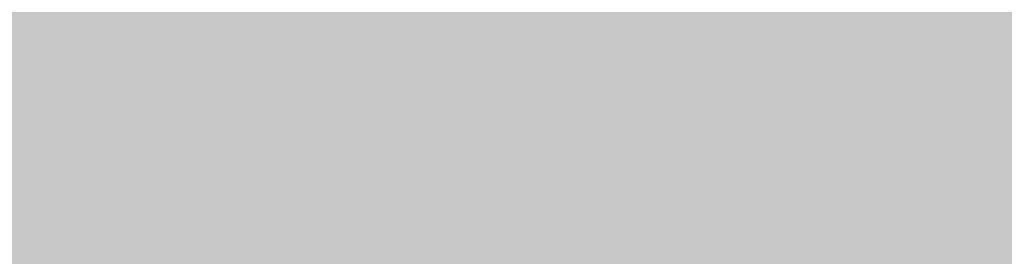
# Model space of a CAD drawing. Units: inches. Extents: x 2083 to 3317, y 1141 to 2115.
# Tile 130 of 256: x 3119.674 to 3123.979, y 1264.131 to 1265.165. Entities that reach past the tile are written whole.
import ezdxf

# ---------------------------------------------------------------- set-up
doc = ezdxf.new("R2010")
doc.units = ezdxf.units.IN
doc.layers.add('A-ANNO-DIMS', color=2, linetype='Continuous', lineweight=18)
doc.layers.add('A-WALL-PATT', color=251, linetype='Continuous', lineweight=13, true_color=0x636466)
doc.styles.get("Standard").update_dxf_attribs({"font": 'arial.ttf'})
doc.dimstyles.new('ISO-25', dxfattribs={"dimtxt": 12, "dimasz": 12, "dimexe": 1.25, "dimexo": 0.625, "dimtad": 1, "dimlunit": 3, "dimtxsty": 'Standard', "dimcen": 2.5, "dimadec": 0, "dimazin": 0, "dimtfac": 1, "dimtmove": 0, "dimatfit": 3, "dimfxl": 1, "dimarcsym": 0})

# ---------------------------------------------------------------- blocks, each defined once
blk = doc.blocks.new('*D26')
at = {"layer": 'A-ANNO-DIMS', "color": 0, "lineweight": -2, "transparency": 16777216}
for p, q in [((3088.9858, 1274.9151), (3088.9858, 1270.952)), ((3111.24, 1274.9151), (3111.24, 1270.952)), ((3076.9858, 1272.202), (2840.2624, 1272.202)), ((3111.24, 1272.202), (3088.9858, 1272.202)), ((3123.24, 1272.202), (3135.24, 1272.202))]:
    blk.add_line(p, q, dxfattribs=at)
at = {"layer": 'A-ANNO-DIMS', "color": 0, "transparency": 16777216}
for points in [[(3076.9858, 1274.202), (3076.9858, 1270.202), (3088.9858, 1272.202)], [(3123.24, 1274.202), (3123.24, 1270.202), (3111.24, 1272.202)]]:
    blk.add_solid(points, dxfattribs=at)
at = {"layer": 'Defpoints', "color": 0, "transparency": 16777216}
for p in [(3088.9858, 1275.5401), (3111.24, 1275.5401), (3088.9858, 1272.202)]:
    blk.add_point(p, dxfattribs=at)
at = {"layer": 'A-ANNO-DIMS', "color": 0, "transparency": 16777216, "insert": (2952.6241, 1279.0316), "char_height": 12, "attachment_point": 5}
blk.add_mtext('NIGHTSTAND 1\'-10 1/2" TYP.', dxfattribs=at)
blk = doc.blocks.new('*D27')
at = {"layer": 'A-ANNO-DIMS', "color": 0, "lineweight": -2, "transparency": 16777216}
for p, q in [((3114.5782, 1309.7943), (3114.5782, 1321.7943)), ((3111.865, 1297.7943), (3115.8282, 1297.7943)), ((3114.5782, 1297.7943), (3114.5782, 1275.5401)), ((3111.865, 1275.5401), (3115.8282, 1275.5401)), ((3114.5782, 1263.5401), (3114.5782, 1140.9886))]:
    blk.add_line(p, q, dxfattribs=at)
at = {"layer": 'A-ANNO-DIMS', "color": 0, "transparency": 16777216}
for points in [[(3112.5782, 1309.7943), (3116.5782, 1309.7943), (3114.5782, 1297.7943)], [(3112.5782, 1263.5401), (3116.5782, 1263.5401), (3114.5782, 1275.5401)]]:
    blk.add_solid(points, dxfattribs=at)
at = {"layer": 'Defpoints', "color": 0, "transparency": 16777216}
for p in [(3111.24, 1297.7943), (3111.24, 1275.5401), (3114.5782, 1275.5401)]:
    blk.add_point(p, dxfattribs=at)
at = {"layer": 'A-ANNO-DIMS', "color": 0, "transparency": 16777216, "insert": (3107.7485, 1196.2643), "char_height": 12, "attachment_point": 5, "rotation": 90}
blk.add_mtext('1\'-10 1/2" TYP.', dxfattribs=at)

msp = doc.modelspace()

# ---------------------------------------------------------------- hatches: boundary and pattern name
at = {"layer": 'A-WALL-PATT'}
h = msp.add_hatch(color=256, dxfattribs=at)
h.dxf.hatch_style = 1
h.paths.add_polyline_path([(3126.9598, 2020.7614), (2748.9598, 2020.7614), (2604.9598, 2020.7614), (2226.9598, 2020.7614), (2226.9598, 1702.7614), (2466.9598, 1702.7614), (2466.9598, 1582.7614), (2418.9598, 1582.7614), (2418.9598, 1477.7614), (2226.9598, 1477.7614), (2226.9598, 1263.2614), (2544.9598, 1263.2614), (2544.9598, 1411.7614), (2604.9598, 1411.7614), (2685.9598, 1411.7614), (2685.9598, 1420.7614), (2604.9598, 1420.7614), (2604.9598, 1573.7614), (2604.9598, 1702.7614), (2604.9598, 2011.7614), (2748.9598, 2011.7614), (2748.9598, 1702.7614), (2862.9598, 1702.7614), (2862.9598, 1621.7614), (2871.9598, 1621.7614), (2871.9598, 1702.7614), (2883.9598, 1702.7614), (2883.9598, 1706.9395, -0.026459), (2883.9598, 1711.7614), (2757.9598, 1711.7614), (2757.9598, 1807.7614), (2787.9598, 1807.7614), (2787.9598, 1812.2614), (2757.9598, 1812.2614), (2757.9598, 2011.7614), (2877.9598, 2011.7614), (2877.9598, 1812.2614), (2847.9598, 1812.2614), (2847.9598, 1807.7614), (2889.8357, 1807.7614), (2889.8357, 1812.2614), (2882.4598, 1812.2614), (2882.4598, 2011.7614), (3117.9598, 2011.7614), (3117.9598, 1812.2614), (2937.8357, 1812.2614), (2937.8357, 1807.7614), (2995.7098, 1807.7614), (2995.7098, 1796.1177), (3000.2098, 1796.1177), (3000.2098, 1807.7614), (3117.9598, 1807.7614), (3117.9598, 1711.7614), (3000.2098, 1711.7614), (3000.2098, 1760.1177), (2998.5727, 1760.1177, -0.020711), (2995.7098, 1760.1177), (2995.7098, 1711.7614), (2931.9598, 1711.7614), (2931.9598, 1702.7614), (3126.9598, 1702.7614)])
h.paths.add_polyline_path([(2471.4598, 2011.7614), (2471.4598, 1810.0114), (2462.7169, 1810.0114), (2462.7169, 1805.5114), (2505.9598, 1805.5114), (2505.9598, 1810.0114), (2475.9598, 1810.0114), (2475.9598, 2011.7614), (2595.9598, 2011.7614), (2595.9598, 1810.0114), (2565.9598, 1810.0114), (2565.9598, 1805.5114), (2595.9598, 1805.5114), (2595.9598, 1711.7614), (2235.9598, 1711.7614), (2235.9598, 1805.5114), (2353.7098, 1805.5114), (2353.7098, 1796.0542), (2358.2098, 1796.0542), (2358.2098, 1805.5114), (2414.7169, 1805.5114), (2414.7169, 1810.0114), (2235.9598, 1810.0114), (2235.9598, 2011.7614)], flags=16)
h.paths.add_polyline_path([(2270.2047, 1994.61), (2270.2047, 1970.61), (2246.2047, 1970.61), (2246.2047, 1994.61)], flags=0)
edge = h.paths.add_edge_path(flags=0)
edge.add_ellipse((2332.0274, 1899.7982), major_axis=(-3.043, 3.043), ratio=0.168252, start_angle=-161.3322, end_angle=-156.3071, ccw=False)
edge.add_ellipse((2333.082, 1898.7435), major_axis=(-1.0546, 1.0546), ratio=0.453532, start_angle=-123.371, end_angle=-94.1591)
edge = h.paths.add_edge_path(flags=0)
edge.add_ellipse((2332.0274, 1968.8763), major_axis=(3.043, 3.043), ratio=0.168252, start_angle=18.6678, end_angle=23.6929)
edge.add_spline(control_points=[(2332.9256, 1970.6911), (2332.2268, 1970.3361), (2330.8937, 1969.6589), (2328.4131, 1970.9321), (2327.2039, 1967.7487), (2324.7096, 1969.9556), (2322.5328, 1967.0124), (2320.0128, 1971.2958), (2317.6803, 1968.1578), (2316.0405, 1967.102), (2315.4269, 1966.8096)], knot_values=[0, 0, 0, 0, 2.267059, 4.324559, 6.685584, 8.878641, 11.121502, 14.300359, 17.755284, 19.732645, 19.732645, 19.732645, 19.732645], degree=3, periodic=0)
edge.add_ellipse((2332.0274, 1968.8763), major_axis=(3.043, 3.043), ratio=0.168252, start_angle=18.6678, end_angle=23.6929, ccw=False)
edge.add_ellipse((2333.082, 1969.9309), major_axis=(1.0546, 1.0546), ratio=0.453532, start_angle=56.629, end_angle=85.8409, ccw=False)
edge = h.paths.add_edge_path(flags=0)
edge.add_spline(control_points=[(2296.4283, 1967.9879), (2293.6278, 1965.3363), (2287.7036, 1959.7271), (2299.7439, 1949.9957), (2294.5326, 1935.6685), (2290.5732, 1920.6035), (2293.3941, 1909.9737), (2296.1854, 1904.9665)], knot_values=[0.099185, 0.099185, 0.099185, 0.099185, 0.345301, 0.619822, 0.982653, 1.386093, 1.810555, 1.810555, 1.810555, 1.810555], degree=3, periodic=0)
edge.add_spline(control_points=[(2296.1854, 1904.9665), (2297.3836, 1902.6193), (2298.001, 1901.9493), (2298.553, 1901.4682)], knot_values=[0.006246, 0.006246, 0.006246, 0.006246, 0.055476, 0.055476, 0.055476, 0.055476], degree=3, periodic=0)
edge.add_spline(control_points=[(2298.553, 1901.4682), (2297.2586, 1900.9232), (2295.2253, 1900.2321), (2293.0602, 1900.6142), (2292.1014, 1900.7884), (2292.0896, 1900.7906)], knot_values=[0.312835, 0.312835, 0.312835, 0.312835, 0.40178, 0.474987, 0.475903, 0.475903, 0.475903, 0.475903], degree=3, periodic=0)
edge.add_arc((2292.7936, 1904.6641), 3.937, 215.4209, 259.6982, ccw=False)
edge.add_spline(control_points=[(2289.5853, 1902.3823), (2289.4767, 1902.5351), (2289.3685, 1902.688), (2289.2609, 1902.8412)], knot_values=[0.102872, 0.102872, 0.102872, 0.102872, 0.116896, 0.116896, 0.116896, 0.116896], degree=3, periodic=0)
edge.add_spline(control_points=[(2289.2609, 1902.8412), (2288.6866, 1902.5502), (2287.64, 1902.0199), (2285.8813, 1901.874), (2283.853, 1901.5044), (2281.72, 1899.7105), (2278.467, 1899.4929), (2276.1571, 1901.8832), (2272.259, 1899.8041), (2267.7776, 1901.8432), (2262.2439, 1900.184), (2257.4149, 1901.7821), (2254.3184, 1900.7261), (2253.1783, 1900.3373)], knot_values=[0, 0, 0, 0, 1.907977, 3.477176, 5.261074, 7.972851, 11.680248, 13.717921, 16.939592, 22.789562, 27.502503, 33.595215, 37.145618, 37.145618, 37.145618, 37.145618], degree=3, periodic=0)
edge.add_line((2253.1783, 1900.3373), (2250.2442, 1902.8412))
edge.add_line((2250.2442, 1902.8412), (2250.2442, 1965.8333))
edge.add_line((2250.2442, 1965.8333), (2253.1783, 1968.3371))
edge.add_spline(control_points=[(2253.1783, 1968.3371), (2254.3184, 1967.9483), (2257.4149, 1966.8924), (2262.2439, 1968.4904), (2267.7776, 1966.8313), (2271.5267, 1968.5372), (2273.8759, 1967.8283), (2274.2067, 1967.7276)], knot_values=[0, 0, 0, 0, 0.09018, 0.244935, 0.364644, 0.513233, 0.537855, 0.537855, 0.537855, 0.537855], degree=3, periodic=0)
edge.add_arc((2274.3529, 1963.7933), 3.937, 72.0511, 92.1279, ccw=False)
edge.add_arc((2281.2969, 1985.23), 18.5963, 252.05113, 288.56572)
edge.add_arc((2292.3167, 1956.0289), 12.6461, 71.02679, 113.77822, ccw=False)
edge = h.paths.add_edge_path(flags=0)
edge.add_spline(control_points=[(2274.8994, 1951.8562), (2275.0662, 1951.6166), (2275.2327, 1951.3766), (2275.398, 1951.1359)], knot_values=[1.409916, 1.409916, 1.409916, 1.409916, 1.43159, 1.43159, 1.43159, 1.43159], degree=3, periodic=0)
edge.add_spline(control_points=[(2275.398, 1951.1359), (2275.7921, 1950.5619), (2276.1792, 1949.9838), (2276.5455, 1949.3971)], knot_values=[1.358238, 1.358238, 1.358238, 1.358238, 1.409916, 1.409916, 1.409916, 1.409916], degree=3, periodic=0)
edge.add_line((2276.5455, 1949.3971), (2277.4373, 1947.8622))
edge.add_spline(control_points=[(2277.4373, 1947.8622), (2276.3038, 1945.6731), (2274.6397, 1942.4269), (2274.6316, 1938.0939), (2272.7991, 1930.8515), (2274.3564, 1943.897), (2275.9477, 1947.9234), (2276.5455, 1949.3971)], knot_values=[0.005632, 0.005632, 0.005632, 0.005632, 0.186014, 0.266002, 0.357087, 0.59639, 0.739732, 0.739732, 0.739732, 0.739732], degree=3, periodic=0)
edge.add_spline(control_points=[(2276.5455, 1949.3971), (2276.1792, 1949.9838), (2275.7921, 1950.5619), (2275.398, 1951.1359)], knot_values=[1.358238, 1.358238, 1.358238, 1.358238, 1.409916, 1.409916, 1.409916, 1.409916], degree=3, periodic=0)
edge.add_spline(control_points=[(2275.398, 1951.1359), (2274.9425, 1950.0805), (2274.2078, 1948.0253), (2273.9346, 1944.8515), (2272.4685, 1937.6275), (2273.4662, 1945.6965), (2274.7006, 1951.0595), (2274.8994, 1951.8562)], knot_values=[0.104364, 0.104364, 0.104364, 0.104364, 0.189636, 0.269624, 0.36071, 0.600013, 0.644622, 0.644622, 0.644622, 0.644622], degree=3, periodic=0)
h.paths.add_polyline_path([(2269.1675, 1963.1276, -0.357527), (2268.1706, 1960.9764, -0.092561), (2268.1706, 1939.4363, -0.357527), (2269.1675, 1937.2851, -0.357527), (2267.0163, 1938.282, -0.164785), (2254.6856, 1938.282, -0.357527), (2252.5344, 1937.2851, -0.357527), (2253.5313, 1939.4363, -0.092561), (2253.5313, 1960.9764, -0.357527), (2252.5344, 1963.1276, -0.357527), (2254.6856, 1962.1307, -0.164785), (2267.0163, 1962.1307, -0.357527)], flags=0)
h.paths.add_polyline_path([(2248.8741, 1967.8018), (2248.8741, 1957.0277), (2249.4578, 1957.0277), (2249.4578, 1911.6468), (2248.8741, 1911.6468), (2248.8741, 1900.8727), (2246.5119, 1900.8727, 0.197327), (2244.1497, 1902.4569), (2244.1497, 1966.2176, 0.197327), (2246.5119, 1967.8018)], flags=0)
h.paths.add_polyline_path([(2269.1675, 1931.3893, -0.357527), (2268.1706, 1929.2381, -0.092561), (2268.1706, 1907.6981, -0.357527), (2269.1675, 1905.5469, -0.357527), (2267.0163, 1906.5438, -0.164785), (2254.6856, 1906.5438, -0.357527), (2252.5344, 1905.5469, -0.357527), (2253.5313, 1907.6981, -0.092561), (2253.5313, 1929.2381, -0.357527), (2252.5344, 1931.3893, -0.357527), (2254.6856, 1930.3925, -0.164785), (2267.0163, 1930.3925, -0.357527)], flags=0)
edge = h.paths.add_edge_path(flags=0)
edge.add_spline(control_points=[(2276.1969, 1906.7237), (2276.1681, 1909.0289), (2276.114, 1913.3719), (2270.5984, 1924.925), (2273.9052, 1919.0128), (2275.9217, 1916.2621), (2275.4746, 1912.4021), (2277.2579, 1910.3806), (2276.696, 1908.225), (2276.6462, 1906.813), (2276.6178, 1906.0084)], knot_values=[0, 0, 0, 0, 8.61026, 16.221274, 18.843057, 23.804898, 27.440828, 29.356102, 31.203478, 33.650687, 33.650687, 33.650687, 33.650687], degree=3, periodic=0)
edge.add_spline(control_points=[(2276.6178, 1906.0084), (2276.6233, 1905.6241), (2276.4977, 1904.6287), (2275.4418, 1903.8547), (2274.9373, 1903.0804), (2274.8591, 1902.8412)], knot_values=[0.156488, 0.156488, 0.156488, 0.156488, 0.184398, 0.231376, 0.250598, 0.250598, 0.250598, 0.250598], degree=3, periodic=0)
edge.add_line((2274.8591, 1902.8412), (2276.506, 1902.8412))
edge.add_spline(control_points=[(2276.506, 1902.8412), (2276.7883, 1903.0849), (2277.6651, 1904.1252), (2278.2495, 1904.3407), (2277.6539, 1908.5274), (2278.1557, 1906.2278), (2278.1005, 1905.2859), (2278.8467, 1904.069), (2277.8568, 1903.4149), (2277.8742, 1902.991), (2277.9036, 1902.8412)], knot_values=[0.059574, 0.059574, 0.059574, 0.059574, 0.080753, 0.103741, 0.16972, 0.176036, 0.207137, 0.240474, 0.262341, 0.27366, 0.27366, 0.27366, 0.27366], degree=3, periodic=0)
edge.add_line((2277.9036, 1902.8412), (2280.0298, 1902.8412))
edge.add_spline(control_points=[(2280.0298, 1902.8412), (2279.8882, 1903.0884), (2279.4993, 1903.9816), (2280.1523, 1905.9393), (2278.1036, 1909.6578), (2279.7624, 1907.1853), (2280.3279, 1904.8749), (2280.4851, 1903.4896), (2281.4633, 1903.2494), (2281.7583, 1902.9365), (2281.834, 1902.8412)], knot_values=[0.013856, 0.013856, 0.013856, 0.013856, 0.034874, 0.088867, 0.107879, 0.126738, 0.158714, 0.193757, 0.217487, 0.226722, 0.226722, 0.226722, 0.226722], degree=3, periodic=0)
edge.add_spline(control_points=[(2281.834, 1902.8412), (2281.7875, 1902.8267), (2281.647, 1902.783), (2281.3955, 1902.8595), (2281.0881, 1902.9852), (2280.7207, 1903.0609), (2280.3335, 1903.0257), (2280.1248, 1902.8989), (2280.0298, 1902.8412)], knot_values=[0, 0, 0, 0, 0.14413, 0.435517, 0.749276, 1.153046, 1.548371, 1.878348, 1.878348, 1.878348, 1.878348], degree=3, periodic=0)
edge.add_line((2280.0298, 1902.8412), (2277.9036, 1902.8412))
edge.add_spline(control_points=[(2277.9036, 1902.8412), (2277.8929, 1902.7959), (2277.8654, 1902.6796), (2277.6075, 1902.6875), (2277.2741, 1902.8007), (2276.8379, 1902.6198), (2276.5838, 1902.7893), (2276.506, 1902.8412)], knot_values=[0, 0, 0, 0, 0.127189, 0.326199, 0.628009, 1.24357, 1.515331, 1.515331, 1.515331, 1.515331], degree=3, periodic=0)
edge.add_line((2276.506, 1902.8412), (2274.8591, 1902.8412))
edge.add_spline(control_points=[(2274.8591, 1902.8412), (2274.8144, 1902.8986), (2274.7251, 1903.0134), (2274.4935, 1903.119), (2274.2443, 1902.9605), (2273.9371, 1903.1849), (2273.614, 1902.9831), (2273.4083, 1902.883), (2273.3223, 1902.8412)], knot_values=[0, 0, 0, 0, 0.21843, 0.436957, 0.687977, 0.990379, 1.398396, 1.69185, 1.69185, 1.69185, 1.69185], degree=3, periodic=0)
edge.add_spline(control_points=[(2273.3223, 1902.8412), (2273.6167, 1903.4457), (2274.274, 1904.5383), (2276.0272, 1904.5737), (2276.207, 1906.5836), (2276.1969, 1906.7237)], knot_values=[0.012227, 0.012227, 0.012227, 0.012227, 0.059472, 0.106218, 0.134458, 0.134458, 0.134458, 0.134458], degree=3, periodic=0)
h.paths.add_polyline_path([(2270.7761, 1897.7898), (2270.7761, 1873.7898), (2246.7761, 1873.7898), (2246.7761, 1897.7898)], flags=0)
h.paths.add_polyline_path([(2353.7098, 1760.0051), (2353.7098, 1760.0542), (2358.2098, 1760.0542, -0.033729)], flags=0)
h.paths.add_polyline_path([(2321.8191, 1737.5292), (2341.9953, 1737.5292, -0.414214), (2343.2033, 1736.3212), (2343.2033, 1721.0206, -0.414214), (2341.9953, 1719.8127), (2321.8191, 1719.8127, -0.414214), (2320.6112, 1721.0206), (2320.6112, 1736.3212, -0.414214)], flags=0)
h.paths.add_polyline_path([(2324.235, 1736.3212), (2339.5794, 1736.3212, -0.414214), (2341.9953, 1733.9053), (2341.9953, 1725.4497, -0.414214), (2339.5794, 1723.0338), (2333.6806, 1723.0338), (2333.8453, 1722.0455, -0.870646), (2335.4254, 1721.8259, -0.767327), (2333.9227, 1721.4232), (2331.291, 1721.4232, -0.767327), (2329.7883, 1721.8259, -0.870646), (2331.3684, 1722.0455), (2331.5331, 1723.0338), (2324.235, 1723.0338, -0.414214), (2321.8191, 1725.4497), (2321.8191, 1733.9053, -0.414214)], flags=0)
h.paths.add_polyline_path([(2570.4838, 1928.6154), (2589.6838, 1928.6154), (2590.1688, 1928.6154), (2590.1688, 1904.9934), (2570.4838, 1904.9934)], flags=0)
h.paths.add_polyline_path([(2574.4473, 1927.2638, -1), (2572.8288, 1927.2638, -1)], flags=0)
h.paths.add_polyline_path([(2573.0899, 1926.9409), (2573.925, 1927.776), (2574.1477, 1927.5533), (2573.3126, 1926.7182)], flags=0)
h.paths.add_polyline_path([(2578.7791, 1919.7296, -1), (2571.5917, 1919.7296, -1)], flags=0)
h.paths.add_polyline_path([(2578.3854, 1919.7296, -1), (2571.9854, 1919.7296, -1)], flags=0)
h.paths.add_polyline_path([(2331.5958, 1729.4762, -1), (2333.618, 1729.4762, -1)], flags=0)
h.paths.add_polyline_path([(2578.0342, 1927.2638, -1), (2576.4157, 1927.2638, -1)], flags=0)
h.paths.add_polyline_path([(2576.6889, 1927.5311), (2576.9116, 1927.7538), (2577.7467, 1926.9186), (2577.524, 1926.6959)], flags=0)
h.paths.add_polyline_path([(2578.1391, 1909.8595, -1), (2572.2317, 1909.8595, -1)], flags=0)
h.paths.add_polyline_path([(2577.7454, 1909.8595, -1), (2572.6254, 1909.8595, -1)], flags=0)
h.paths.add_polyline_path([(2583.7977, 1927.2638, -1), (2582.1792, 1927.2638, -1)], flags=0)
h.paths.add_polyline_path([(2582.7186, 1927.7538), (2583.5538, 1926.9186), (2583.3311, 1926.6959), (2582.4959, 1927.5311)], flags=0)
h.paths.add_polyline_path([(2582.4959, 1927.5311), (2582.7186, 1927.7538), (2583.5538, 1926.9186), (2583.3311, 1926.6959)], flags=0)
h.paths.add_polyline_path([(2587.7391, 1920.5296, -1), (2581.8317, 1920.5296, -1)], flags=0)
h.paths.add_polyline_path([(2587.3454, 1920.5296, -1), (2582.2254, 1920.5296, -1)], flags=0)
h.paths.add_polyline_path([(2587.3846, 1927.2638, -1), (2585.7661, 1927.2638, -1)], flags=0)
h.paths.add_polyline_path([(2586.082, 1926.9802), (2586.9172, 1927.8154), (2587.1399, 1927.5927), (2586.3047, 1926.7575)], flags=0)
h.paths.add_polyline_path([(2588.3791, 1910.6595, -1), (2581.1917, 1910.6595, -1)], flags=0)
h.paths.add_polyline_path([(2587.9854, 1910.6595, -1), (2581.5854, 1910.6595, -1)], flags=0)
h.paths.add_polyline_path([(2417.1677, 1729.4779), (2437.3439, 1729.4779, -0.414214), (2438.5519, 1728.2699), (2438.5519, 1712.9693, -0.414214), (2437.3439, 1711.7614), (2417.1677, 1711.7614, -0.414214), (2415.9598, 1712.9693), (2415.9598, 1728.2699, -0.414214)], flags=0)
h.paths.add_polyline_path([(2419.5836, 1728.2699), (2434.928, 1728.2699, -0.414214), (2437.3439, 1725.8541), (2437.3439, 1717.3984, -0.414214), (2434.928, 1714.9825), (2429.0292, 1714.9825), (2429.1939, 1713.9942, -0.870646), (2430.774, 1713.7746, -0.767327), (2429.2713, 1713.372), (2426.6396, 1713.372, -0.767327), (2425.1369, 1713.7746, -0.870646), (2426.717, 1713.9942), (2426.8817, 1714.9825), (2419.5836, 1714.9825, -0.414214), (2417.1677, 1717.3984), (2417.1677, 1725.8541, -0.414214)], flags=0)
h.paths.add_polyline_path([(2419.5836, 1728.2699), (2434.928, 1728.2699, -0.414214), (2437.3439, 1725.8541), (2437.3439, 1717.3984, -0.414214), (2434.928, 1714.9825), (2429.0292, 1714.9825), (2428.3581, 1719.009), (2427.5528, 1719.009), (2426.8817, 1714.9825), (2419.5836, 1714.9825, -0.414214), (2417.1677, 1717.3984), (2417.1677, 1725.8541, -0.414214)], flags=0)
h.paths.add_polyline_path([(2426.9444, 1721.4249, -1), (2428.9666, 1721.4249, -1)], flags=0)
h.paths.add_polyline_path([(2475.9598, 1702.7614), (2595.9598, 1702.7614), (2595.9598, 1582.7614), (2475.9598, 1582.7614)], flags=16)
h.paths.add_polyline_path([(2427.9598, 1573.7614), (2595.9598, 1573.7614), (2595.9598, 1468.7614), (2595.9598, 1420.7614), (2384.4598, 1420.7614), (2384.4598, 1468.7614), (2427.9598, 1468.7614)], flags=16)
h.paths.add_polyline_path([(2379.9598, 1468.7614), (2379.9598, 1420.7614), (2235.9598, 1420.7614), (2235.9598, 1468.7614)], flags=16)
h.paths.add_polyline_path([(2317.816, 1466.6958), (2337.9922, 1466.6958, -0.414214), (2339.2002, 1465.4878), (2339.2002, 1450.1872, -0.414214), (2337.9922, 1448.9792), (2317.816, 1448.9792, -0.414214), (2316.6081, 1450.1872), (2316.6081, 1465.4878, -0.414214)], flags=0)
h.paths.add_polyline_path([(2320.2319, 1465.4878), (2335.5763, 1465.4878, -0.414214), (2337.9922, 1463.0719), (2337.9922, 1454.6163, -0.414214), (2335.5763, 1452.2004), (2329.6775, 1452.2004), (2329.8422, 1451.212, -0.870646), (2331.4223, 1450.9925, -0.767327), (2329.9196, 1450.5898), (2327.2879, 1450.5898, -0.767327), (2325.7852, 1450.9925, -0.870646), (2327.3653, 1451.212), (2327.53, 1452.2004), (2320.2319, 1452.2004, -0.414214), (2317.816, 1454.6163), (2317.816, 1463.0719, -0.414214)], flags=0)
h.paths.add_polyline_path([(2320.2319, 1465.4878), (2335.5763, 1465.4878, -0.414214), (2337.9922, 1463.0719), (2337.9922, 1454.6163, -0.414214), (2335.5763, 1452.2004), (2329.6775, 1452.2004), (2329.0064, 1456.2269), (2328.2011, 1456.2269), (2327.53, 1452.2004), (2320.2319, 1452.2004, -0.414214), (2317.816, 1454.6163), (2317.816, 1463.0719, -0.414214)], flags=0)
h.paths.add_polyline_path([(2327.5926, 1458.6428, -1), (2329.6148, 1458.6428, -1)], flags=0)
h.paths.add_polyline_path([(2244.4117, 1433.3405), (2241.9209, 1433.3405, -0.414214), (2240.0179, 1435.2435), (2240.0179, 1440.9528, -0.414211), (2241.9209, 1442.8559), (2244.4117, 1442.8559, -1.976472)], flags=0)
h.paths.add_polyline_path([(2245.3569, 1434.3975, -0.414214), (2245.3569, 1441.7988, -2.144098)], flags=0)
h.paths.add_polyline_path([(2535.9598, 1416.2614), (2535.9598, 1272.2614), (2235.9598, 1272.2614), (2235.9598, 1416.2614)], flags=16)
h.paths.add_polyline_path([(2260.1196, 1384.2928), (2260.1196, 1362.0386), (2237.8654, 1362.0386), (2237.8654, 1384.2928)], flags=0)
edge = h.paths.add_edge_path(flags=0)
edge.add_line((2318.2518, 1362.0933), (2318.1458, 1362.001))
edge.add_ellipse((2317.4451, 1360.431), major_axis=(2.8216, 2.8216), ratio=0.168252, start_angle=18.6678, end_angle=20.9481, ccw=False)
edge.add_ellipse((2318.423, 1361.409), major_axis=(0.9779, 0.9779), ratio=0.453532, start_angle=56.629, end_angle=70.2262, ccw=False)
edge = h.paths.add_edge_path(flags=0)
edge.add_line((2319.1074, 1295.5711), (2319.015, 1295.6771))
edge.add_ellipse((2317.4451, 1296.3778), major_axis=(-2.8216, 2.8216), ratio=0.168252, start_angle=-161.3322, end_angle=-159.0519, ccw=False)
edge.add_ellipse((2318.423, 1295.3999), major_axis=(-0.9779, 0.9779), ratio=0.453532, start_angle=-123.371, end_angle=-109.7738)
edge = h.paths.add_edge_path(flags=0)
edge.add_spline(control_points=[(2284.2103, 1301.1702), (2284.5807, 1300.4447), (2284.8912, 1299.892), (2285.1596, 1299.461)], knot_values=[0.039066, 0.039066, 0.039066, 0.039066, 0.055476, 0.055476, 0.055476, 0.055476], degree=3, periodic=0)
edge.add_line((2285.1596, 1299.461), (2284.2103, 1301.1702))
edge = h.paths.add_edge_path(flags=0)
edge.add_line((2280.4125, 1297.298), (2283.37, 1297.0361))
edge.add_line((2283.37, 1297.0361), (2286.4057, 1297.9263))
edge.add_spline(control_points=[(2286.4057, 1297.9263), (2285.3055, 1297.4631), (2284.3448, 1297.1292), (2283.37, 1297.0361)], knot_values=[0.394369, 0.394369, 0.394369, 0.394369, 0.475903, 0.475903, 0.475903, 0.475903], degree=3, periodic=0)
edge.add_spline(control_points=[(2283.37, 1297.0361), (2283.2814, 1297.0277), (2282.3163, 1296.9573), (2281.3125, 1297.1345), (2280.4234, 1297.296), (2280.4125, 1297.298)], knot_values=[0.312835, 0.312835, 0.312835, 0.312835, 0.320246, 0.393453, 0.394369, 0.394369, 0.394369, 0.394369], degree=3, periodic=0)
edge = h.paths.add_edge_path(flags=0)
edge.add_line((2284.4356, 1359.6073), (2280.4463, 1355.328))
edge.add_line((2280.4463, 1355.328), (2279.58, 1351.0178))
edge.add_line((2279.58, 1351.0178), (2282.413, 1346.5804))
edge.add_spline(control_points=[(2282.413, 1346.5804), (2283.1533, 1345.5892), (2284.2529, 1344.0289), (2284.801, 1342.3872), (2284.9352, 1341.8055)], knot_values=[1.240098, 1.240098, 1.240098, 1.240098, 1.332892, 1.382712, 1.382712, 1.382712, 1.382712], degree=3, periodic=0)
edge.add_spline(control_points=[(2284.9352, 1341.8055), (2285.3191, 1340.1406), (2285.233, 1338.4092), (2284.9099, 1336.6541)], knot_values=[1.097484, 1.097484, 1.097484, 1.097484, 1.240098, 1.240098, 1.240098, 1.240098], degree=3, periodic=0)
edge.add_spline(control_points=[(2284.9099, 1336.6541), (2284.5868, 1334.899), (2284.0267, 1333.1203), (2283.4626, 1331.3606)], knot_values=[0.95487, 0.95487, 0.95487, 0.95487, 1.097484, 1.097484, 1.097484, 1.097484], degree=3, periodic=0)
edge.add_line((2283.4626, 1331.3606), (2281.8904, 1326.1534))
edge.add_line((2281.8904, 1326.1534), (2280.7563, 1321.0561))
edge.add_line((2280.7563, 1321.0561), (2280.2992, 1316.002))
edge.add_line((2280.2992, 1316.002), (2280.7159, 1310.9501))
edge.add_line((2280.7159, 1310.9501), (2282.0281, 1305.9721))
edge.add_line((2282.0281, 1305.9721), (2284.2103, 1301.1702))
edge.add_spline(control_points=[(2284.2103, 1301.1702), (2283.3407, 1302.7302), (2282.6119, 1304.3365), (2282.0281, 1305.9721)], knot_values=[0.099185, 0.099185, 0.099185, 0.099185, 0.241799, 0.241799, 0.241799, 0.241799], degree=3, periodic=0)
edge.add_spline(control_points=[(2282.0281, 1305.9721), (2281.4443, 1307.6078), (2281.0055, 1309.2728), (2280.7159, 1310.9501)], knot_values=[0.241799, 0.241799, 0.241799, 0.241799, 0.384413, 0.384413, 0.384413, 0.384413], degree=3, periodic=0)
edge.add_spline(control_points=[(2280.7159, 1310.9501), (2280.4332, 1312.5876), (2280.2894, 1314.277), (2280.2989, 1315.962), (2280.2992, 1316.002)], knot_values=[0.384413, 0.384413, 0.384413, 0.384413, 0.523647, 0.527028, 0.527028, 0.527028, 0.527028], degree=3, periodic=0)
edge.add_spline(control_points=[(2280.2992, 1316.002), (2280.3123, 1317.687), (2280.4779, 1319.3679), (2280.7563, 1321.0561)], knot_values=[0.527028, 0.527028, 0.527028, 0.527028, 0.669642, 0.669642, 0.669642, 0.669642], degree=3, periodic=0)
edge.add_spline(control_points=[(2280.7563, 1321.0561), (2281.0346, 1322.7443), (2281.4259, 1324.4396), (2281.8904, 1326.1534)], knot_values=[0.669642, 0.669642, 0.669642, 0.669642, 0.812256, 0.812256, 0.812256, 0.812256], degree=3, periodic=0)
edge.add_spline(control_points=[(2281.8904, 1326.1534), (2282.2644, 1327.5333), (2282.7879, 1329.2618), (2283.3528, 1331.0178), (2283.4626, 1331.3606)], knot_values=[0.812256, 0.812256, 0.812256, 0.812256, 0.927087, 0.95487, 0.95487, 0.95487, 0.95487], degree=3, periodic=0)
edge.add_line((2283.4626, 1331.3606), (2284.9099, 1336.6541))
edge.add_line((2284.9099, 1336.6541), (2284.9352, 1341.8055))
edge.add_line((2284.9352, 1341.8055), (2282.413, 1346.5804))
edge.add_spline(control_points=[(2282.413, 1346.5804), (2281.2751, 1348.1038), (2280.0784, 1349.5703), (2279.58, 1351.0178)], knot_values=[1.382712, 1.382712, 1.382712, 1.382712, 1.525326, 1.525326, 1.525326, 1.525326], degree=3, periodic=0)
edge.add_spline(control_points=[(2279.58, 1351.0178), (2279.4433, 1351.4147), (2279.1363, 1352.8569), (2279.7352, 1354.2904), (2280.4463, 1355.328)], knot_values=[1.525326, 1.525326, 1.525326, 1.525326, 1.564439, 1.667941, 1.667941, 1.667941, 1.667941], degree=3, periodic=0)
edge.add_spline(control_points=[(2280.4463, 1355.328), (2281.4261, 1356.7578), (2282.9308, 1358.1826), (2284.4356, 1359.6073)], knot_values=[1.667941, 1.667941, 1.667941, 1.667941, 1.810555, 1.810555, 1.810555, 1.810555], degree=3, periodic=0)
edge.add_arc((2280.6231, 1348.5182), 11.7262, 71.02679, 113.77822)
edge.add_arc((2270.4049, 1375.5952), 17.2436, 252.05113, 288.56572, ccw=False)
edge.add_arc((2263.966, 1355.7178), 3.6506, 72.0511, 92.1279)
edge.add_arc((2263.966, 1355.7178), 3.6506, 92.1279, 177.9851)
edge.add_spline(control_points=[(2260.3176, 1355.8462), (2260.2604, 1354.2207), (2260.5513, 1350.1865), (2262.9993, 1346.7663), (2264.4727, 1344.649)], knot_values=[1.43159, 1.43159, 1.43159, 1.43159, 1.564144, 1.770695, 1.770695, 1.770695, 1.770695], degree=3, periodic=0)
edge.add_line((2264.4727, 1344.649), (2264.9356, 1343.9825))
edge.add_spline(control_points=[(2263.801, 1340.2481), (2263.8432, 1340.5141), (2264.0672, 1341.7565), (2264.5127, 1343.0025), (2264.935, 1343.9811)], knot_values=[0.53657, 0.53657, 0.53657, 0.53657, 0.559349, 0.644622, 0.644622, 0.644622, 0.644622], degree=3, periodic=0)
edge.add_spline(control_points=[(2264.935, 1343.9811), (2265.1178, 1343.715), (2265.2989, 1343.4479), (2265.4768, 1343.1794)], knot_values=[1.384077, 1.384077, 1.384077, 1.384077, 1.409916, 1.409916, 1.409916, 1.409916], degree=3, periodic=0)
edge.add_spline(control_points=[(2265.4768, 1343.1794), (2265.6546, 1342.9108), (2265.8293, 1342.6408), (2265.9991, 1342.3688)], knot_values=[1.358238, 1.358238, 1.358238, 1.358238, 1.384077, 1.384077, 1.384077, 1.384077], degree=3, periodic=0)
edge.add_line((2265.9991, 1342.3688), (2266.826, 1340.9455))
edge.add_spline(control_points=[(2266.826, 1340.9455), (2268.8944, 1337.0897), (2271.3982, 1325.843), (2270.5162, 1310.5686), (2275.9194, 1301.8606), (2277.7895, 1299.1994)], knot_values=[0.116896, 0.116896, 0.116896, 0.116896, 0.472987, 1.050969, 1.313793, 1.313793, 1.313793, 1.313793], degree=3, periodic=0)
edge.add_spline(control_points=[(2277.7895, 1299.1994), (2277.8394, 1299.1285), (2277.8894, 1299.0575), (2277.9396, 1298.9866)], knot_values=[0.109884, 0.109884, 0.109884, 0.109884, 0.116896, 0.116896, 0.116896, 0.116896], degree=3, periodic=0)
edge.add_line((2277.9396, 1298.9866), (2277.7888, 1299.1991))
edge.add_spline(control_points=[(2277.7888, 1299.1991), (2277.2566, 1298.9294), (2276.2864, 1298.4379), (2275.0394, 1298.3344), (2274.3833, 1298.2389), (2274.2153, 1298.2093)], knot_values=[33.12187, 33.12187, 33.12187, 33.12187, 35.029056, 36.598255, 37.144827, 37.144827, 37.144827, 37.144827], degree=3, periodic=0)
edge.add_line((2274.2153, 1298.2093), (2273.0731, 1297.893))
edge.add_spline(control_points=[(2273.0731, 1297.893), (2272.3229, 1297.5798), (2271.0392, 1296.5105), (2269.2484, 1296.2261), (2268.4231, 1296.3747)], knot_values=[26.532584, 26.532584, 26.532584, 26.532584, 29.198919, 31.839101, 31.839101, 31.839101, 31.839101], degree=3, periodic=0)
edge.add_line((2268.4231, 1296.3747), (2263.8785, 1297.4575))
edge.add_spline(control_points=[(2263.8785, 1297.4575), (2263.5561, 1297.3594), (2261.8603, 1296.8387), (2260.2388, 1297.2824), (2258.9335, 1297.5165)], knot_values=[15.919551, 15.919551, 15.919551, 15.919551, 16.939592, 21.226067, 21.226067, 21.226067, 21.226067], degree=3, periodic=0)
edge.add_line((2258.9335, 1297.5165), (2254.0552, 1297.329))
edge.add_spline(control_points=[(2254.0552, 1297.329), (2253.7555, 1297.2958), (2252.1137, 1297.1652), (2250.4619, 1297.5442), (2249.1297, 1297.6679)], knot_values=[5.306517, 5.306517, 5.306517, 5.306517, 6.276435, 10.613034, 10.613034, 10.613034, 10.613034], degree=3, periodic=0)
edge.add_line((2249.1297, 1297.6679), (2244.3316, 1296.8778))
edge.add_line((2244.3316, 1296.8778), (2241.611, 1299.1994))
edge.add_line((2241.611, 1299.1994), (2241.611, 1357.6094))
edge.add_line((2241.611, 1357.6094), (2244.3316, 1359.9311))
edge.add_line((2244.3316, 1359.9311), (2252.7288, 1359.5427))
edge.add_spline(control_points=[(2252.7288, 1359.5427), (2252.8709, 1359.5464), (2253.3057, 1359.5482), (2253.7398, 1359.5143), (2254.0317, 1359.4824)], knot_values=[0.233291, 0.233291, 0.233291, 0.233291, 0.244935, 0.268927, 0.268927, 0.268927, 0.268927], degree=3, periodic=0)
edge.add_line((2254.0317, 1359.4824), (2259.5872, 1359.4164))
edge.add_spline(control_points=[(2259.5872, 1359.4164), (2260.6771, 1359.6285), (2262.0732, 1359.897), (2263.5237, 1359.4593), (2263.8304, 1359.366)], knot_values=[0.422516, 0.422516, 0.422516, 0.422516, 0.513233, 0.537855, 0.537855, 0.537855, 0.537855], degree=3, periodic=0)
edge.add_arc((2263.966, 1355.7178), 3.6506, 72.0511, 92.1279, ccw=False)
edge.add_arc((2270.4049, 1375.5952), 17.2436, 252.05113, 288.56572)
edge.add_arc((2280.6231, 1348.5182), 11.7262, 71.02679, 113.77822, ccw=False)
h.paths.add_polyline_path([(2240.3405, 1359.4347), (2240.3405, 1349.4444), (2240.8818, 1349.4444), (2240.8818, 1307.3645), (2240.3405, 1307.3645), (2240.3405, 1297.3741), (2238.1502, 1297.3741, 0.197327), (2235.9598, 1298.8431), (2235.9598, 1357.9657, 0.197327), (2238.1502, 1359.4347)], flags=0)
h.paths.add_polyline_path([(2259.1578, 1355.1005, -0.357527), (2258.2334, 1353.1058, -0.092561), (2258.2334, 1333.1326, -0.357527), (2259.1578, 1331.1379, -0.357527), (2257.1631, 1332.0622, -0.164785), (2245.7293, 1332.0622, -0.357527), (2243.7346, 1331.1379, -0.357527), (2244.6589, 1333.1326, -0.092561), (2244.6589, 1353.1058, -0.357527), (2243.7346, 1355.1005, -0.357527), (2245.7293, 1354.1761, -0.164785), (2257.1631, 1354.1761, -0.357527)], flags=0)
edge = h.paths.add_edge_path(flags=0)
edge.add_line((2265.9991, 1342.3688), (2266.826, 1340.9455))
edge.add_line((2266.826, 1340.9455), (2265.3076, 1337.8141))
edge.add_line((2265.3076, 1337.8141), (2264.3582, 1334.6529))
edge.add_line((2264.3582, 1334.6529), (2264.262, 1333.7997))
edge.add_spline(control_points=[(2264.262, 1333.7997), (2264.2084, 1333.1871), (2264.1621, 1332.3655), (2264.0071, 1331.4139), (2263.969, 1331.2018)], knot_values=[0.464444, 0.464444, 0.464444, 0.464444, 0.516691, 0.531608, 0.531608, 0.531608, 0.531608], degree=3, periodic=0)
edge.add_spline(control_points=[(2263.969, 1331.2018), (2263.7745, 1330.1189), (2263.4244, 1328.7908), (2263.2574, 1328.5307), (2263.234, 1328.5146)], knot_values=[0.372682, 0.372682, 0.372682, 0.372682, 0.44885, 0.464444, 0.464444, 0.464444, 0.464444], degree=3, periodic=0)
edge.add_spline(control_points=[(2263.234, 1328.5146), (2263.0964, 1328.4202), (2263.1312, 1329.3015), (2263.275, 1330.6157)], knot_values=[0.280919, 0.280919, 0.280919, 0.280919, 0.372682, 0.372682, 0.372682, 0.372682], degree=3, periodic=0)
edge.add_spline(control_points=[(2263.275, 1330.6157), (2263.4187, 1331.93), (2263.6715, 1333.6773), (2263.9699, 1335.315)], knot_values=[0.189157, 0.189157, 0.189157, 0.189157, 0.280919, 0.280919, 0.280919, 0.280919], degree=3, periodic=0)
edge.add_spline(control_points=[(2263.9699, 1335.315), (2264.1005, 1336.0322), (2264.4188, 1337.6219), (2264.7548, 1338.8644), (2264.9474, 1339.4911)], knot_values=[0.097394, 0.097394, 0.097394, 0.097394, 0.137578, 0.189157, 0.189157, 0.189157, 0.189157], degree=3, periodic=0)
edge.add_spline(control_points=[(2264.9474, 1339.4911), (2265.29, 1340.6061), (2265.6442, 1341.494), (2265.9991, 1342.3688)], knot_values=[0.005632, 0.005632, 0.005632, 0.005632, 0.097394, 0.097394, 0.097394, 0.097394], degree=3, periodic=0)
h.paths.add_polyline_path([(2259.1578, 1325.671, -0.357527), (2258.2334, 1323.6763, -0.092561), (2258.2334, 1303.7031, -0.357527), (2259.1578, 1301.7084, -0.357527), (2257.1631, 1302.6327, -0.164785), (2245.7293, 1302.6327, -0.357527), (2243.7346, 1301.7084, -0.357527), (2244.6589, 1303.7031, -0.092561), (2244.6589, 1323.6763, -0.357527), (2243.7346, 1325.671, -0.357527), (2245.7293, 1324.7466, -0.164785), (2257.1631, 1324.7466, -0.357527)], flags=0)
edge = h.paths.add_edge_path(flags=0)
edge.add_spline(control_points=[(2261.7089, 1317.3114), (2261.6795, 1317.4176), (2261.7619, 1317.3885), (2262.4907, 1316.0899), (2262.9622, 1315.3009)], knot_values=[14.955861, 14.955861, 14.955861, 14.955861, 16.221274, 18.694826, 18.694826, 18.694826, 18.694826], degree=3, periodic=0)
edge.add_spline(control_points=[(2262.9622, 1315.3009), (2262.9904, 1315.2536), (2263.7021, 1314.0674), (2264.349, 1313.1272), (2264.7301, 1312.1642)], knot_values=[18.694826, 18.694826, 18.694826, 18.694826, 18.843057, 22.433791, 22.433791, 22.433791, 22.433791], degree=3, periodic=0)
edge.add_spline(control_points=[(2264.7301, 1312.1642), (2264.8756, 1311.7964), (2265.1769, 1310.7698), (2265.1431, 1309.5593), (2265.2477, 1308.8242)], knot_values=[22.433791, 22.433791, 22.433791, 22.433791, 23.804898, 26.172756, 26.172756, 26.172756, 26.172756], degree=3, periodic=0)
edge.add_line((2265.2477, 1308.8242), (2265.8508, 1307.1719))
edge.add_spline(control_points=[(2265.8508, 1307.1719), (2266.065, 1306.8217), (2266.3844, 1306.3322), (2266.4244, 1305.7805), (2266.4204, 1305.6112)], knot_values=[28.062562, 28.062562, 28.062562, 28.062562, 29.356102, 29.911721, 29.911721, 29.911721, 29.911721], degree=3, periodic=0)
edge.add_spline(control_points=[(2266.4204, 1305.6112), (2266.4161, 1305.4326), (2266.394, 1305.25), (2266.3648, 1305.0659)], knot_values=[29.911721, 29.911721, 29.911721, 29.911721, 30.497837, 30.497837, 30.497837, 30.497837], degree=3, periodic=0)
edge.add_line((2266.3648, 1305.0659), (2266.0662, 1302.1363))
edge.add_spline(control_points=[(2266.0662, 1302.1363), (2266.0712, 1301.78), (2265.9981, 1301.2), (2265.6633, 1300.759), (2265.5089, 1300.5859)], knot_values=[0.156488, 0.156488, 0.156488, 0.156488, 0.184398, 0.203543, 0.203543, 0.203543, 0.203543], degree=3, periodic=0)
edge.add_line((2265.5089, 1300.5859), (2264.4353, 1299.1994))
edge.add_line((2264.4353, 1299.1994), (2265.9624, 1299.1994))
edge.add_line((2265.9624, 1299.1994), (2267.336, 1301.1753))
edge.add_line((2267.336, 1301.1753), (2267.3117, 1301.9862))
edge.add_spline(control_points=[(2267.3117, 1301.9862), (2267.2611, 1302.8624), (2267.1602, 1303.7371), (2267.2715, 1303.3259)], knot_values=[0.126229, 0.126229, 0.126229, 0.126229, 0.166617, 0.166617, 0.166617, 0.166617], degree=3, periodic=0)
edge.add_spline(control_points=[(2267.2715, 1303.3259), (2267.28, 1303.2943), (2267.3098, 1303.1754), (2267.3735, 1302.8836), (2267.4061, 1302.6828), (2267.4179, 1302.601)], knot_values=[0.166617, 0.166617, 0.166617, 0.166617, 0.16972, 0.176036, 0.180765, 0.180765, 0.180765, 0.180765], degree=3, periodic=0)
edge.add_spline(control_points=[(2267.7439, 1300.9875), (2267.6876, 1301.1509), (2267.4805, 1301.6567), (2267.4838, 1302.1448), (2267.4179, 1302.601)], knot_values=[0.180765, 0.180765, 0.180765, 0.180765, 0.193767, 0.220139, 0.220139, 0.220139, 0.220139], degree=3, periodic=0)
edge.add_line((2267.4179, 1302.601), (2267.7439, 1300.9875))
edge.add_spline(control_points=[(2267.7439, 1300.9875), (2267.832, 1300.7319), (2267.932, 1300.3099), (2267.5548, 1299.9745), (2267.4294, 1299.8292)], knot_values=[0.220139, 0.220139, 0.220139, 0.220139, 0.240474, 0.25489, 0.25489, 0.25489, 0.25489], degree=3, periodic=0)
edge.add_line((2267.4294, 1299.8292), (2267.2584, 1299.1994))
edge.add_line((2267.2584, 1299.1994), (2269.23, 1299.1994))
edge.add_spline(control_points=[(2269.23, 1299.1994), (2269.0987, 1299.4287), (2268.8428, 1300.0163), (2269.0116, 1300.9159), (2268.9468, 1301.6607)], knot_values=[0.013856, 0.013856, 0.013856, 0.013856, 0.034874, 0.067073, 0.067073, 0.067073, 0.067073], degree=3, periodic=0)
edge.add_line((2268.9468, 1301.6607), (2268.4316, 1303.6031))
edge.add_spline(control_points=[(2268.4316, 1303.6031), (2268.1756, 1304.1924), (2267.5962, 1305.2513), (2268.0407, 1304.6232), (2268.2514, 1304.2824)], knot_values=[0.090155, 0.090155, 0.090155, 0.090155, 0.107879, 0.120289, 0.120289, 0.120289, 0.120289], degree=3, periodic=0)
edge.add_spline(control_points=[(2268.2514, 1304.2824), (2268.3609, 1304.1053), (2269.0578, 1302.918), (2269.3827, 1301.5904), (2269.5214, 1300.7759), (2269.5752, 1300.5558)], knot_values=[0.120289, 0.120289, 0.120289, 0.120289, 0.126738, 0.158714, 0.173506, 0.173506, 0.173506, 0.173506], degree=3, periodic=0)
edge.add_line((2269.5752, 1300.5558), (2270.6858, 1299.4213))
edge.add_spline(control_points=[(2270.6858, 1299.4213), (2270.7672, 1299.3573), (2270.8379, 1299.2814), (2270.9029, 1299.1994)], knot_values=[0.21816, 0.21816, 0.21816, 0.21816, 0.226722, 0.226722, 0.226722, 0.226722], degree=3, periodic=0)
edge.add_line((2270.9372, 1299.1929), (2270.9029, 1299.1994))
edge.add_spline(control_points=[(2270.9029, 1299.1994), (2270.8598, 1299.186), (2270.7295, 1299.1455), (2270.4963, 1299.2164), (2270.2717, 1299.3083), (2270.121, 1299.348), (2270.0633, 1299.3596)], knot_values=[0.939174, 0.939174, 0.939174, 0.939174, 1.083304, 1.374691, 1.68845, 1.878348, 1.878348, 1.878348, 1.878348], degree=3, periodic=0)
edge.add_line((2270.0633, 1299.3596), (2269.23, 1299.1994))
edge.add_line((2269.23, 1299.1994), (2267.2584, 1299.1994))
edge.add_spline(control_points=[(2267.2584, 1299.1994), (2267.2484, 1299.1574), (2267.223, 1299.0497), (2266.9838, 1299.0569), (2266.8092, 1299.1162), (2266.6769, 1299.1091), (2266.6365, 1299.1048)], knot_values=[0.757665, 0.757665, 0.757665, 0.757665, 0.884854, 1.083864, 1.385675, 1.515331, 1.515331, 1.515331, 1.515331], degree=3, periodic=0)
edge.add_spline(control_points=[(2266.6365, 1299.1048), (2266.4852, 1299.0888), (2266.2358, 1299.0171), (2266.0346, 1299.1513), (2265.9624, 1299.1994)], knot_values=[0, 0, 0, 0, 0.485905, 0.757665, 0.757665, 0.757665, 0.757665], degree=3, periodic=0)
edge.add_line((2265.9624, 1299.1994), (2264.4353, 1299.1994))
edge.add_line((2264.4353, 1299.1994), (2263.8584, 1299.3671))
edge.add_spline(control_points=[(2263.8584, 1299.3671), (2263.8189, 1299.3709), (2263.7795, 1299.3857), (2263.7401, 1299.4015)], knot_values=[0.845925, 0.845925, 0.845925, 0.845925, 0.978627, 0.978627, 0.978627, 0.978627], degree=3, periodic=0)
edge.add_line((2263.7218, 1299.3964), (2263.0103, 1299.1994))
edge.add_spline(control_points=[(2263.0103, 1299.1994), (2263.2458, 1299.6829), (2263.506, 1300.1281), (2263.8735, 1300.408)], knot_values=[0.012227, 0.012227, 0.012227, 0.012227, 0.052971, 0.052971, 0.052971, 0.052971], degree=3, periodic=0)
edge.add_spline(control_points=[(2263.8735, 1300.408), (2263.9321, 1300.4527), (2264.0842, 1300.553), (2264.2552, 1300.6242), (2264.3597, 1300.6647)], knot_values=[0.052971, 0.052971, 0.052971, 0.052971, 0.059472, 0.069086, 0.069086, 0.069086, 0.069086], degree=3, periodic=0)
edge.add_line((2264.3597, 1300.6647), (2265.1419, 1301.0778))
edge.add_line((2265.1419, 1301.0778), (2265.6758, 1302.7996))
edge.add_line((2265.6758, 1302.7996), (2265.5407, 1305.7041))
edge.add_line((2265.5407, 1305.7041), (2264.8031, 1309.3277))
edge.add_line((2264.8031, 1309.3277), (2263.0405, 1314.0918))
edge.add_spline(control_points=[(2263.0405, 1314.0918), (2262.3836, 1315.6714), (2261.796, 1316.9977), (2261.7089, 1317.3114)], knot_values=[11.216896, 11.216896, 11.216896, 11.216896, 14.955861, 14.955861, 14.955861, 14.955861], degree=3, periodic=0)
h.paths.add_polyline_path([(2871.9598, 1416.2614), (2895.91, 1416.2614), (2895.91, 1420.7614), (2871.9598, 1420.7614), (2871.9598, 1501.7614), (2862.9598, 1501.7614), (2862.9598, 1420.7614), (2805.9598, 1420.7614), (2805.9598, 1411.7614), (2862.9598, 1411.7614), (2862.9598, 1263.2614), (3126.9598, 1263.2614), (3126.9598, 1411.7614), (3126.9598, 1486.7614), (2943.9598, 1486.7614), (2943.9598, 1477.7614), (2967.8603, 1477.7614), (2967.8603, 1420.7614), (2943.91, 1420.7614), (2943.91, 1416.2614), (3117.9598, 1416.2614), (3117.9598, 1420.7614), (2972.3603, 1420.7614), (2972.3603, 1477.7614), (3117.9598, 1477.7614), (3117.9598, 1420.7614), (3117.9598, 1272.2614), (2871.9598, 1272.2614)], flags=0)
h.paths.add_polyline_path([(2457.1256, 1485.9425), (2527.6027, 1485.9425), (2527.6027, 1537.6357), (2457.1256, 1537.6357)], flags=8)
h.paths.add_polyline_path([(2481.0051, 1609.9818), (2590.7658, 1609.9818), (2590.7658, 1682.0034), (2481.0051, 1682.0034)], flags=8)
h.paths.add_polyline_path([(2483.085, 1729.1268), (2553.562, 1729.1268), (2553.562, 1780.82), (2483.085, 1780.82)], flags=8)
h = msp.add_hatch(color=256, dxfattribs=at)
h.dxf.hatch_style = 1
h.paths.add_polyline_path([(3126.9598, 1486.7614), (2943.9598, 1486.7614), (2943.9598, 1477.7614), (2967.8603, 1477.7614), (2967.8603, 1420.7614), (2943.91, 1420.7614), (2943.91, 1416.2614), (3117.9598, 1416.2614), (3117.9598, 1420.7614), (2972.3603, 1420.7614), (2972.3603, 1477.7614), (3117.9598, 1477.7614), (3117.9598, 1420.7614), (3117.9598, 1272.2614), (2871.9598, 1272.2614), (2871.9598, 1416.2614), (2895.91, 1416.2614), (2895.91, 1420.7614), (2871.9598, 1420.7614), (2871.9598, 1501.7614), (2862.9598, 1501.7614), (2862.9598, 1420.7614), (2805.9598, 1420.7614), (2805.9598, 1411.7614), (2862.9598, 1411.7614), (2862.9598, 1263.2614), (3126.9598, 1263.2614), (3126.9598, 1411.7614)])

# ---------------------------------------------------------------- dimensions: what is measured, and where the dimension line sits
at = {"layer": 'A-ANNO-DIMS'}
for base, p1, p2, angle, text, picture, middle in [((3114.5782, 1275.5401), (3111.24, 1297.7943), (3111.24, 1275.5401), 270, '<> TYP.', '*D27', (3107.7485, 1196.2643)), ((3088.9858, 1272.202), (3111.24, 1275.5401), (3088.9858, 1275.5401), 180, 'NIGHTSTAND <> TYP.', '*D26', (2952.6241, 1279.0316))]:
    dim = msp.add_linear_dim(base=base, p1=p1, p2=p2, angle=angle, text=text, dimstyle='ISO-25', override={"dimdec": 1, "dimlfac": 1, "dimrnd": 0, "dimzin": 1, "dimdsep": 46, "dimlunit": 4, "dimfrac": 2}, dxfattribs=at)
    dim.commit()
    dim.dimension.update_dxf_attribs({"geometry": picture, "text_midpoint": middle})

doc.saveas('drawing.dxf')
